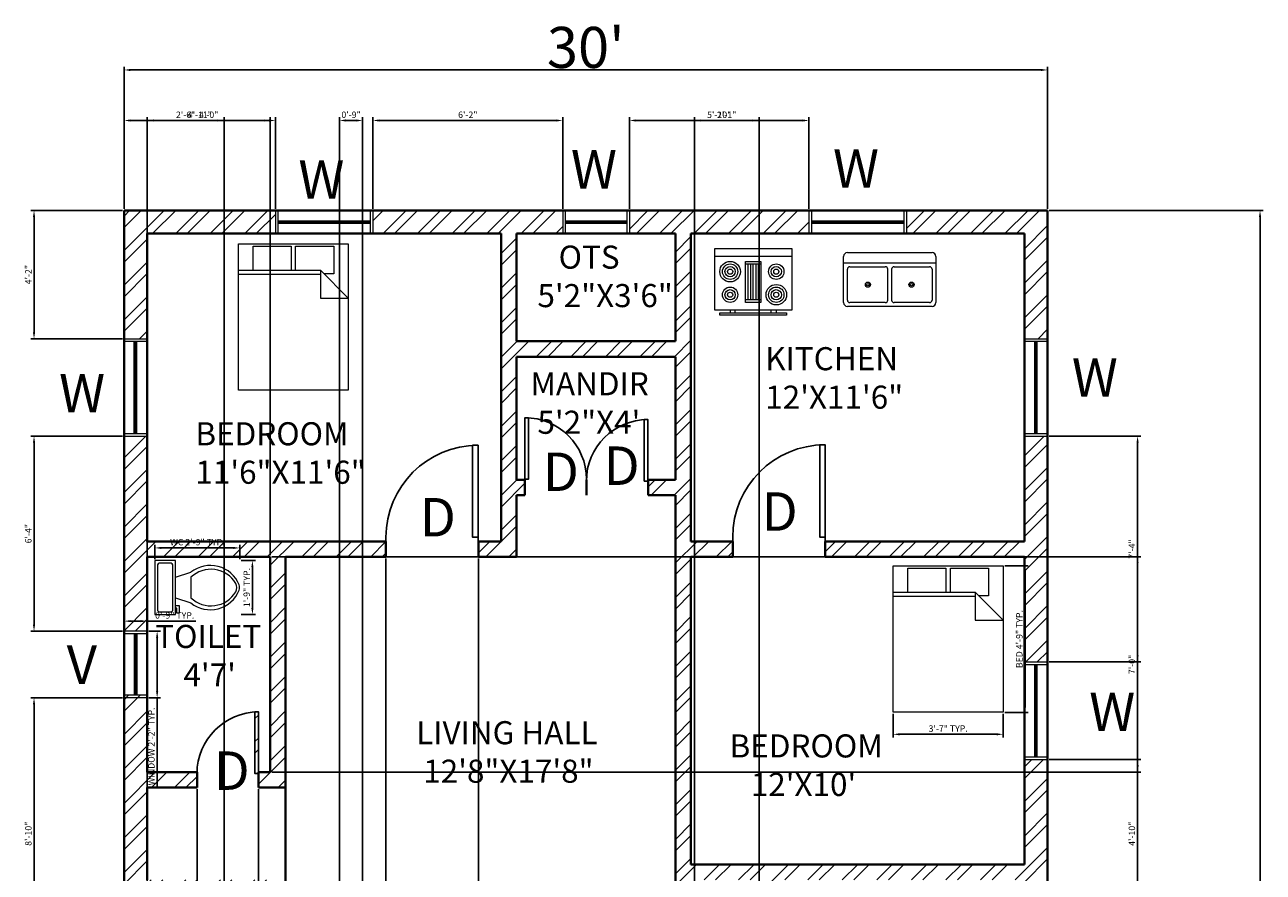
# Model space of a CAD drawing. Units: inches. Extents: x 1143 to 1626, y 7431 to 8140.
# Tile 4 of 4: x 1143 to 1626, y 7809 to 8140. Entities that reach past the tile are written whole.
import ezdxf

# ---------------------------------------------------------------- set-up
doc = ezdxf.new("R2010")
doc.units = ezdxf.units.IN
for name, color, linetype, lineweight in [('A-ANNO-DIMS', 4, 'Continuous', 18), ('A-DOOR', 3, 'Continuous', 25), ('A-GLAZ', 4, 'Continuous', 18), ('A-WALL', 2, 'Continuous', 40), ('A-WALL-PATT', 7, 'Continuous', 13)]:
    doc.layers.add(name, color=color, linetype=linetype, lineweight=lineweight)
for name, color, linetype, lineweight, true_color in [('A-ANNO-TEXT', 40, 'Continuous', 18, 0xf8d731), ('A-AREA-IDEN', 40, 'Continuous', 25, 0xf8d731), ('A-EQPM', 40, 'Continuous', 18, 0xf8d731), ('A-FLOR-FIXT', 40, 'Continuous', 18, 0xf8d731), ('A-FURN', 40, 'Continuous', 18, 0xf8d731)]:
    doc.layers.add(name, color=color, linetype=linetype, lineweight=lineweight, true_color=true_color)
doc.styles.get("Standard").update_dxf_attribs({"font": 'arial.ttf'})
doc.dimstyles.new('ISO-25', dxfattribs={"dimtxt": 2.5, "dimasz": 2.5, "dimexe": 1.25, "dimexo": 0.625, "dimtad": 1, "dimdec": 0, "dimlunit": 3, "dimtxsty": 'Standard', "dimcen": 2.5, "dimadec": 0, "dimazin": 0, "dimtfac": 1, "dimtdec": 0, "dimtmove": 0, "dimatfit": 3, "dimfxl": 1, "dimarcsym": 0})

# ---------------------------------------------------------------- blocks, each defined once
blk = doc.blocks.new('*U8')
for p, q in [((0, 0), (0, -100)), ((750, 0), (750, -100))]:
    blk.add_line(p, q)
blk.add_lwpolyline([(0, 0), (0, 750), (43.75, 750), (43.75, 0)], close=True)
blk.add_arc((0, 0), 750, 0, 90)
blk = doc.blocks.new('Bed - Queen')
for p, q in [((0, -80.00003), (0, 0)), ((0, 0), (59.99999, 0)), ((59.99999, 0), (59.99999, -80.00003)), ((7.99999, -1.2), (28.79998, -1.2)), ((7.99999, -14.4), (7.99999, -1.2)), ((28.79998, -1.2), (28.79998, -14.4)), ((31.19999, -1.2), (51.99999, -1.2)), ((31.19999, -14.4), (31.19999, -1.2)), ((51.99999, -1.2), (51.99999, -16.4)), ((0, -14.4), (44.8, -14.4)), ((44.8, -16.8), (0, -16.8)), ((59.99999, -29.6), (44.8, -14.4)), ((44.8, -14.4), (44.8, -29.6)), ((51.99999, -16.4), (46.79936, -16.4)), ((44.8, -29.6), (59.99999, -29.6)), ((59.99999, -80.00003), (0, -80.00003))]:
    blk.add_line(p, q)
blk = doc.blocks.new('Toilet - top')
for p, q in [((9.5, -6), (9.5, -2)), ((-10, -8.5), (-8, -8.5)), ((-10, -9.5), (-10, -8.5)), ((-7, -9.5), (-10, -9.5)), ((-8, -8.5), (-8, -8)), ((-7, -8), (-7, -9.5)), ((-4, -8), (-6, -14)), ((4, -8), (6, -14)), ((4, -14), (-4, -14))]:
    blk.add_line(p, q)
blk.add_lwpolyline([(10.5, -8), (10.5, 0), (-10.5, 0), (-10.5, -8)], close=True)
for points in [[(-9.5, -2), (-9.5, -6)], [(8.5, -1), (-8.5, -1)], [(-8.5, -7), (8.5, -7)]]:
    blk.add_lwpolyline(points)
for centre, radius, start, end in [((-8.62, -1.88), 0.884, 81.8699, 188.1301), ((8.62, -1.88), 0.884, 351.8699, 98.1301), ((-8.62, -6.12), 0.884, 171.8699, 278.1301), ((8.62, -6.12), 0.884, 261.8699, 8.1301), ((3.52, -21.58), 12.17, 141.4691, 247.9714), ((4.2, -21.82), 11.33, 136.3677, 238.9468), ((-3.52, -21.58), 12.17, 292.0284, 38.5307), ((-4.2, -21.82), 11.33, 301.053, 43.6321), ((0, -27.88), 4, 245.7318, 294.2682), ((0, -29), 4, 254.8605, 285.1395)]:
    blk.add_arc(centre, radius, start, end)
blk = doc.blocks.new('Range-Oven - 30 in top')
for p, q in [((0, -3), (30, -3)), ((12, -6), (18, -6)), ((13, -20), (13, -6)), ((14, -6), (14, -20)), ((15, -20), (15, -6)), ((16, -6), (16, -20)), ((17, -20), (17, -6)), ((6, -24), (6, -25)), ((8, -25), (8, -24)), ((18, -20), (12, -20)), ((22, -25), (22, -24)), ((24, -24), (24, -25))]:
    blk.add_line(p, q)
for points in [[(0, -24), (0, 0), (30, 0), (30, -24)], [(12, -21), (12, -5), (18, -5), (18, -21)], [(2, -26), (2, -25), (28, -25), (28, -26)]]:
    blk.add_lwpolyline(points, close=True)
for centre, radius in [((6, -9), 4), ((6, -9), 3), ((6, -9), 2), ((6, -9), 1), ((24, -9), 3), ((24, -9), 2), ((24, -9), 1), ((24, -18), 4), ((6, -18), 3), ((6, -18), 2), ((6, -18), 1), ((24, -18), 3), ((24, -18), 2), ((24, -18), 1)]:
    blk.add_circle(centre, radius)
blk = doc.blocks.new('Sink-double - 36 in top')
for p, q in [((-18, -4), (18, -4)), ((-0.75, -18.5), (-0.75, -6.5)), ((0.75, -6.5), (0.75, -18.5))]:
    blk.add_line(p, q)
for points in [[(-16.5, 0), (16.5, 0)], [(-18, -19.5), (-18, -1.5)], [(18, -1.5), (18, -19.5)], [(-16.5, -18.5), (-16.5, -6.5)], [(-15.5, -5.5), (-1.75, -5.5)], [(1.75, -5.5), (15.5, -5.5)], [(16.5, -6.5), (16.5, -18.5)], [(16.5, -21), (-16.5, -21)], [(-1.75, -19.5), (-15.5, -19.5)], [(15.5, -19.5), (1.75, -19.5)]]:
    blk.add_lwpolyline(points)
for centre, radius in [((-8.5, -12.5), 1), ((-8.5, -12.5), 0.5), ((8.5, -12.5), 1), ((8.5, -12.5), 0.5)]:
    blk.add_circle(centre, radius)
for centre, radius, start, end in [((-16.5, -1.5), 1.5, 90, 180), ((16.5, -1.5), 1.5, 0, 90), ((-15.5, -6.5), 1, 90, 180), ((-1.75, -6.5), 1, 0, 90), ((1.75, -6.5), 1, 90, 180), ((15.5, -6.5), 1, 0, 90), ((-15.5, -18.5), 1, 180, 270), ((-1.75, -18.5), 1, 270, 0), ((1.75, -18.5), 1, 180, 270), ((15.5, -18.5), 1, 270, 0), ((-16.5, -19.5), 1.5, 180, 270), ((16.5, -19.5), 1.5, 270, 0)]:
    blk.add_arc(centre, radius, start, end)
blk = doc.blocks.new('*D58')
at = {"layer": 'A-ANNO-DIMS', "color": 0, "lineweight": -2, "transparency": 16777216}
for p, q in [((1181.85, 8068.02), (1181.85, 8123.44)), ((1184.35, 8122.19), (1539.35, 8122.19)), ((1541.85, 8068.02), (1541.85, 8123.44))]:
    blk.add_line(p, q, dxfattribs=at)
at = {"layer": 'A-ANNO-DIMS', "color": 0, "transparency": 16777216}
for points in [[(1184.35, 8122.61), (1184.35, 8121.77), (1181.85, 8122.19)], [(1539.35, 8122.61), (1539.35, 8121.77), (1541.85, 8122.19)]]:
    blk.add_solid(points, dxfattribs=at)
at = {"layer": 'Defpoints', "color": 0, "transparency": 16777216}
for p in [(1541.85, 8122.19), (1181.85, 8067.4), (1541.85, 8067.4)]:
    blk.add_point(p, dxfattribs=at)
at = {"layer": 'A-ANNO-DIMS', "color": 0, "transparency": 16777216, "insert": (1361.85, 8130.99), "char_height": 2.5, "attachment_point": 5}
blk.add_mtext("{\\H6.4x;30'}", dxfattribs=at)
blk = doc.blocks.new('*D59')
at = {"layer": 'A-ANNO-DIMS', "color": 0, "lineweight": -2, "transparency": 16777216}
for p, q in [((1542.48, 8067.4), (1625.93, 8067.4)), ((1624.68, 8064.9), (1624.68, 7469.9)), ((1542.48, 7467.4), (1625.93, 7467.4))]:
    blk.add_line(p, q, dxfattribs=at)
at = {"layer": 'A-ANNO-DIMS', "color": 0, "transparency": 16777216}
for points in [[(1624.27, 8064.9), (1625.1, 8064.9), (1624.68, 8067.4)], [(1624.27, 7469.9), (1625.1, 7469.9), (1624.68, 7467.4)]]:
    blk.add_solid(points, dxfattribs=at)
at = {"layer": 'Defpoints', "color": 0, "transparency": 16777216}
for p in [(1541.85, 8067.4), (1541.85, 7467.4), (1624.68, 7467.4)]:
    blk.add_point(p, dxfattribs=at)
at = {"layer": 'A-ANNO-DIMS', "color": 0, "transparency": 16777216, "insert": (1615.89, 7767.4), "char_height": 2.5, "attachment_point": 5, "rotation": 90}
blk.add_mtext("{\\H6.4x;50'}", dxfattribs=at)
blk = doc.blocks.new('WIN-36IN')
for p, q in [((0, 9), (0, 0)), ((1, 9), (1, 0)), ((1, 5), (37, 5)), ((37, 9), (37, 0)), ((38, 9), (38, 0)), ((1, 4.5), (37, 4.5)), ((1, 4), (37, 4))]:
    blk.add_line(p, q)
blk = doc.blocks.new('WIN-24IN')
for p, q in [((0, 9), (0, 0)), ((1, 9), (1, 0)), ((1, 5), (25, 5)), ((25, 9), (25, 0)), ((26, 9), (26, 0)), ((1, 4.5), (25, 4.5)), ((1, 4), (25, 4))]:
    blk.add_line(p, q)
blk = doc.blocks.new('*D64')
at = {"layer": 'A-ANNO-DIMS', "color": 0, "lineweight": -2, "transparency": 16777216}
for p, q in [((1191.48, 7903.4), (1196, 7903.4)), ((1194.75, 7900.9), (1194.75, 7879.9)), ((1191.48, 7877.4), (1196, 7877.4)), ((1194.75, 7877.4), (1194.75, 7842.01))]:
    blk.add_line(p, q, dxfattribs=at)
at = {"layer": 'A-ANNO-DIMS', "color": 0, "transparency": 16777216}
for points in [[(1194.33, 7900.9), (1195.17, 7900.9), (1194.75, 7903.4)], [(1194.33, 7879.9), (1195.17, 7879.9), (1194.75, 7877.4)]]:
    blk.add_solid(points, dxfattribs=at)
at = {"layer": 'Defpoints', "color": 0, "transparency": 16777216}
for p in [(1190.85, 7903.4), (1190.85, 7877.4), (1194.75, 7877.4)]:
    blk.add_point(p, dxfattribs=at)
at = {"layer": 'A-ANNO-DIMS', "color": 0, "transparency": 16777216, "insert": (1192.83, 7858.45), "char_height": 2.5, "attachment_point": 5, "rotation": 90}
blk.add_mtext('WINDOW 2\'-2" TYP.', dxfattribs=at)
blk = doc.blocks.new('*D65')
at = {"layer": 'A-ANNO-DIMS', "color": 0, "lineweight": -2, "transparency": 16777216}
for p, q in [((1181.85, 7904.02), (1181.85, 7908.55)), ((1190.85, 7904.02), (1190.85, 7908.55)), ((1184.35, 7907.3), (1188.35, 7907.3)), ((1190.85, 7907.3), (1209.84, 7907.3))]:
    blk.add_line(p, q, dxfattribs=at)
at = {"layer": 'A-ANNO-DIMS', "color": 0, "transparency": 16777216}
for points in [[(1184.35, 7907.71), (1184.35, 7906.88), (1181.85, 7907.3)], [(1188.35, 7907.71), (1188.35, 7906.88), (1190.85, 7907.3)]]:
    blk.add_solid(points, dxfattribs=at)
at = {"layer": 'Defpoints', "color": 0, "transparency": 16777216}
for p in [(1181.85, 7903.4), (1190.85, 7907.3), (1190.85, 7903.4)]:
    blk.add_point(p, dxfattribs=at)
at = {"layer": 'A-ANNO-DIMS', "color": 0, "transparency": 16777216, "insert": (1201.59, 7909.2), "char_height": 2.5, "attachment_point": 5}
blk.add_mtext('0\'-9" TYP.', dxfattribs=at)
blk = doc.blocks.new('*D66')
at = {"layer": 'A-ANNO-DIMS', "color": 0, "lineweight": -2, "transparency": 16777216}
for p, q in [((1193.88, 7931.51), (1193.88, 7937.09)), ((1226.93, 7931.51), (1226.93, 7937.09)), ((1224.43, 7935.84), (1196.38, 7935.84))]:
    blk.add_line(p, q, dxfattribs=at)
at = {"layer": 'A-ANNO-DIMS', "color": 0, "transparency": 16777216}
for points in [[(1196.38, 7936.26), (1196.38, 7935.42), (1193.88, 7935.84)], [(1224.43, 7936.26), (1224.43, 7935.42), (1226.93, 7935.84)]]:
    blk.add_solid(points, dxfattribs=at)
at = {"layer": 'Defpoints', "color": 0, "transparency": 16777216}
for p in [(1193.88, 7935.84), (1193.88, 7930.88), (1226.93, 7930.88)]:
    blk.add_point(p, dxfattribs=at)
at = {"layer": 'A-ANNO-DIMS', "color": 0, "transparency": 16777216, "insert": (1210.41, 7937.76), "char_height": 2.5, "attachment_point": 5}
blk.add_mtext('WC 2\'-9" TYP.', dxfattribs=at)
blk = doc.blocks.new('*D67')
at = {"layer": 'A-ANNO-DIMS', "color": 0, "lineweight": -2, "transparency": 16777216}
for p, q in [((1227.56, 7930.88), (1233.14, 7930.88)), ((1231.89, 7912.38), (1231.89, 7928.38)), ((1227.56, 7909.88), (1233.14, 7909.88))]:
    blk.add_line(p, q, dxfattribs=at)
at = {"layer": 'A-ANNO-DIMS', "color": 0, "transparency": 16777216}
for points in [[(1231.47, 7928.38), (1232.3, 7928.38), (1231.89, 7930.88)], [(1231.47, 7912.38), (1232.3, 7912.38), (1231.89, 7909.88)]]:
    blk.add_solid(points, dxfattribs=at)
at = {"layer": 'Defpoints', "color": 0, "transparency": 16777216}
for p in [(1226.93, 7930.88), (1231.89, 7930.88), (1226.93, 7909.88)]:
    blk.add_point(p, dxfattribs=at)
at = {"layer": 'A-ANNO-DIMS', "color": 0, "transparency": 16777216, "insert": (1229.99, 7920.38), "char_height": 2.5, "attachment_point": 5, "rotation": 90}
blk.add_mtext('1\'-9" TYP.', dxfattribs=at)
blk = doc.blocks.new('*D68')
at = {"layer": 'A-ANNO-DIMS', "color": 0, "lineweight": -2, "transparency": 16777216}
for p, q in [((1525.14, 7928.84), (1534.33, 7928.84)), ((1533.08, 7874.24), (1533.08, 7926.34)), ((1525.14, 7871.74), (1534.33, 7871.74))]:
    blk.add_line(p, q, dxfattribs=at)
at = {"layer": 'A-ANNO-DIMS', "color": 0, "transparency": 16777216}
for points in [[(1532.67, 7926.34), (1533.5, 7926.34), (1533.08, 7928.84)], [(1532.67, 7874.24), (1533.5, 7874.24), (1533.08, 7871.74)]]:
    blk.add_solid(points, dxfattribs=at)
at = {"layer": 'Defpoints', "color": 0, "transparency": 16777216}
for p in [(1524.52, 7928.84), (1533.08, 7928.84), (1524.52, 7871.74)]:
    blk.add_point(p, dxfattribs=at)
at = {"layer": 'A-ANNO-DIMS', "color": 0, "transparency": 16777216, "insert": (1531.18, 7900.29), "char_height": 2.5, "attachment_point": 5, "rotation": 90}
blk.add_mtext('BED 4\'-9" TYP.', dxfattribs=at)
blk = doc.blocks.new('*D69')
at = {"layer": 'A-ANNO-DIMS', "color": 0, "lineweight": -2, "transparency": 16777216}
for p, q in [((1481.7, 7871.12), (1481.7, 7861.93)), ((1524.52, 7871.12), (1524.52, 7861.93)), ((1484.2, 7863.18), (1522.02, 7863.18))]:
    blk.add_line(p, q, dxfattribs=at)
at = {"layer": 'A-ANNO-DIMS', "color": 0, "transparency": 16777216}
for points in [[(1484.2, 7863.6), (1484.2, 7862.76), (1481.7, 7863.18)], [(1522.02, 7863.6), (1522.02, 7862.76), (1524.52, 7863.18)]]:
    blk.add_solid(points, dxfattribs=at)
at = {"layer": 'Defpoints', "color": 0, "transparency": 16777216}
for p in [(1481.7, 7871.74), (1524.52, 7871.74), (1524.52, 7863.18)]:
    blk.add_point(p, dxfattribs=at)
at = {"layer": 'A-ANNO-DIMS', "color": 0, "transparency": 16777216, "insert": (1503.11, 7865.08), "char_height": 2.5, "attachment_point": 5}
blk.add_mtext('3\'-7" TYP.', dxfattribs=at)
blk = doc.blocks.new('*D85')
at = {"layer": 'A-ANNO-DIMS', "color": 0, "lineweight": -2, "transparency": 16777216}
for p, q in [((1283.96, 7931.77), (1283.96, 7431.05)), ((1319.96, 7931.77), (1319.96, 7431.05)), ((1286.46, 7432.3), (1317.46, 7432.3))]:
    blk.add_line(p, q, dxfattribs=at)
at = {"layer": 'A-ANNO-DIMS', "color": 0, "transparency": 16777216}
for points in [[(1286.46, 7432.71), (1286.46, 7431.88), (1283.96, 7432.3)], [(1317.46, 7432.71), (1317.46, 7431.88), (1319.96, 7432.3)]]:
    blk.add_solid(points, dxfattribs=at)
at = {"layer": 'Defpoints', "color": 0, "transparency": 16777216}
for p in [(1283.96, 7932.4), (1319.96, 7932.4), (1319.96, 7432.3)]:
    blk.add_point(p, dxfattribs=at)
at = {"layer": 'A-ANNO-DIMS', "color": 0, "transparency": 16777216, "insert": (1301.96, 7434.2), "char_height": 2.5, "attachment_point": 5}
blk.add_mtext('3\'-0"', dxfattribs=at)
blk = doc.blocks.new('*D86')
at = {"layer": 'A-ANNO-DIMS', "color": 0, "lineweight": -2, "transparency": 16777216}
for p, q in [((1210.31, 7841.77), (1210.31, 7431.05)), ((1234.31, 7841.77), (1234.31, 7431.05)), ((1212.81, 7432.3), (1231.81, 7432.3))]:
    blk.add_line(p, q, dxfattribs=at)
at = {"layer": 'A-ANNO-DIMS', "color": 0, "transparency": 16777216}
for points in [[(1212.81, 7432.71), (1212.81, 7431.88), (1210.31, 7432.3)], [(1231.81, 7432.71), (1231.81, 7431.88), (1234.31, 7432.3)]]:
    blk.add_solid(points, dxfattribs=at)
at = {"layer": 'Defpoints', "color": 0, "transparency": 16777216}
for p in [(1210.31, 7842.4), (1234.31, 7842.4), (1234.31, 7432.3)]:
    blk.add_point(p, dxfattribs=at)
at = {"layer": 'A-ANNO-DIMS', "color": 0, "transparency": 16777216, "insert": (1222.31, 7434.2), "char_height": 2.5, "attachment_point": 5}
blk.add_mtext('2\'-0"', dxfattribs=at)
blk = doc.blocks.new('*D87')
at = {"layer": 'A-ANNO-DIMS', "color": 0, "lineweight": -2, "transparency": 16777216}
for p, q in [((1181.85, 8068.02), (1181.85, 8103.75)), ((1184.35, 8102.5), (1238.35, 8102.5)), ((1240.85, 8068.02), (1240.85, 8103.75))]:
    blk.add_line(p, q, dxfattribs=at)
at = {"layer": 'A-ANNO-DIMS', "color": 0, "transparency": 16777216}
for points in [[(1184.35, 8102.91), (1184.35, 8102.08), (1181.85, 8102.5)], [(1238.35, 8102.91), (1238.35, 8102.08), (1240.85, 8102.5)]]:
    blk.add_solid(points, dxfattribs=at)
at = {"layer": 'Defpoints', "color": 0, "transparency": 16777216}
for p in [(1240.85, 8102.5), (1181.85, 8067.4), (1240.85, 8067.4)]:
    blk.add_point(p, dxfattribs=at)
at = {"layer": 'A-ANNO-DIMS', "color": 0, "transparency": 16777216, "insert": (1211.35, 8104.38), "char_height": 2.5, "attachment_point": 5}
blk.add_mtext('4\'-11"', dxfattribs=at)
blk = doc.blocks.new('*D88')
at = {"layer": 'A-ANNO-DIMS', "color": 0, "lineweight": -2, "transparency": 16777216}
for p, q in [((1278.85, 8068.02), (1278.85, 8103.75)), ((1281.35, 8102.5), (1350.35, 8102.5)), ((1352.85, 8068.02), (1352.85, 8103.75))]:
    blk.add_line(p, q, dxfattribs=at)
at = {"layer": 'A-ANNO-DIMS', "color": 0, "transparency": 16777216}
for points in [[(1281.35, 8102.91), (1281.35, 8102.08), (1278.85, 8102.5)], [(1350.35, 8102.91), (1350.35, 8102.08), (1352.85, 8102.5)]]:
    blk.add_solid(points, dxfattribs=at)
at = {"layer": 'Defpoints', "color": 0, "transparency": 16777216}
for p in [(1352.85, 8102.5), (1278.85, 8067.4), (1352.85, 8067.4)]:
    blk.add_point(p, dxfattribs=at)
at = {"layer": 'A-ANNO-DIMS', "color": 0, "transparency": 16777216, "insert": (1315.85, 8104.4), "char_height": 2.5, "attachment_point": 5}
blk.add_mtext('6\'-2"', dxfattribs=at)
blk = doc.blocks.new('*D89')
at = {"layer": 'A-ANNO-DIMS', "color": 0, "lineweight": -2, "transparency": 16777216}
for p, q in [((1378.85, 8068.02), (1378.85, 8103.75)), ((1381.35, 8102.5), (1446.35, 8102.5)), ((1448.85, 8068.02), (1448.85, 8103.75))]:
    blk.add_line(p, q, dxfattribs=at)
at = {"layer": 'A-ANNO-DIMS', "color": 0, "transparency": 16777216}
for points in [[(1381.35, 8102.91), (1381.35, 8102.08), (1378.85, 8102.5)], [(1446.35, 8102.91), (1446.35, 8102.08), (1448.85, 8102.5)]]:
    blk.add_solid(points, dxfattribs=at)
at = {"layer": 'Defpoints', "color": 0, "transparency": 16777216}
for p in [(1448.85, 8102.5), (1378.85, 8067.4), (1448.85, 8067.4)]:
    blk.add_point(p, dxfattribs=at)
at = {"layer": 'A-ANNO-DIMS', "color": 0, "transparency": 16777216, "insert": (1413.85, 8104.4), "char_height": 2.5, "attachment_point": 5}
blk.add_mtext('5\'-10"', dxfattribs=at)
blk = doc.blocks.new('*D90')
at = {"layer": 'A-ANNO-DIMS', "color": 0, "lineweight": -2, "transparency": 16777216}
for p, q in [((1181.23, 8067.4), (1145.5, 8067.4)), ((1146.75, 8019.9), (1146.75, 8064.9)), ((1181.23, 8017.4), (1145.5, 8017.4))]:
    blk.add_line(p, q, dxfattribs=at)
at = {"layer": 'A-ANNO-DIMS', "color": 0, "transparency": 16777216}
for points in [[(1146.33, 8064.9), (1147.17, 8064.9), (1146.75, 8067.4)], [(1146.33, 8019.9), (1147.17, 8019.9), (1146.75, 8017.4)]]:
    blk.add_solid(points, dxfattribs=at)
at = {"layer": 'Defpoints', "color": 0, "transparency": 16777216}
for p in [(1146.75, 8067.4), (1181.85, 8067.4), (1181.85, 8017.4)]:
    blk.add_point(p, dxfattribs=at)
at = {"layer": 'A-ANNO-DIMS', "color": 0, "transparency": 16777216, "insert": (1144.87, 8042.4), "char_height": 2.5, "attachment_point": 5, "rotation": 90}
blk.add_mtext('4\'-2"', dxfattribs=at)
blk = doc.blocks.new('*D92')
at = {"layer": 'A-ANNO-DIMS', "color": 0, "lineweight": -2, "transparency": 16777216}
for p, q in [((1181.23, 7877.4), (1145.5, 7877.4)), ((1146.75, 7773.9), (1146.75, 7874.9)), ((1181.23, 7771.4), (1145.5, 7771.4))]:
    blk.add_line(p, q, dxfattribs=at)
at = {"layer": 'A-ANNO-DIMS', "color": 0, "transparency": 16777216}
for points in [[(1146.33, 7874.9), (1147.17, 7874.9), (1146.75, 7877.4)], [(1146.33, 7773.9), (1147.17, 7773.9), (1146.75, 7771.4)]]:
    blk.add_solid(points, dxfattribs=at)
at = {"layer": 'Defpoints', "color": 0, "transparency": 16777216}
for p in [(1146.75, 7877.4), (1181.85, 7877.4), (1181.85, 7771.4)]:
    blk.add_point(p, dxfattribs=at)
at = {"layer": 'A-ANNO-DIMS', "color": 0, "transparency": 16777216, "insert": (1144.85, 7824.4), "char_height": 2.5, "attachment_point": 5, "rotation": 90}
blk.add_mtext('8\'-10"', dxfattribs=at)
blk = doc.blocks.new('*D93')
at = {"layer": 'A-ANNO-DIMS', "color": 0, "lineweight": -2, "transparency": 16777216}
for p, q in [((1181.23, 7979.4), (1145.5, 7979.4)), ((1146.75, 7905.9), (1146.75, 7976.9)), ((1181.23, 7903.4), (1145.5, 7903.4))]:
    blk.add_line(p, q, dxfattribs=at)
at = {"layer": 'A-ANNO-DIMS', "color": 0, "transparency": 16777216}
for points in [[(1146.33, 7976.9), (1147.17, 7976.9), (1146.75, 7979.4)], [(1146.33, 7905.9), (1147.17, 7905.9), (1146.75, 7903.4)]]:
    blk.add_solid(points, dxfattribs=at)
at = {"layer": 'Defpoints', "color": 0, "transparency": 16777216}
for p in [(1146.75, 7979.4), (1181.85, 7979.4), (1181.85, 7903.4)]:
    blk.add_point(p, dxfattribs=at)
at = {"layer": 'A-ANNO-DIMS', "color": 0, "transparency": 16777216, "insert": (1144.85, 7941.4), "char_height": 2.5, "attachment_point": 5, "rotation": 90}
blk.add_mtext('6\'-4"', dxfattribs=at)
blk = doc.blocks.new('*D96')
at = {"layer": 'A-ANNO-DIMS', "color": 0, "lineweight": -2, "transparency": 16777216}
for p, q in [((1542.48, 7853.4), (1578.2, 7853.4)), ((1576.95, 7797.9), (1576.95, 7850.9)), ((1542.48, 7795.4), (1578.2, 7795.4))]:
    blk.add_line(p, q, dxfattribs=at)
at = {"layer": 'A-ANNO-DIMS', "color": 0, "transparency": 16777216}
for points in [[(1576.53, 7850.9), (1577.37, 7850.9), (1576.95, 7853.4)], [(1576.53, 7797.9), (1577.37, 7797.9), (1576.95, 7795.4)]]:
    blk.add_solid(points, dxfattribs=at)
at = {"layer": 'Defpoints', "color": 0, "transparency": 16777216}
for p in [(1541.85, 7853.4), (1576.95, 7853.4), (1541.85, 7795.4)]:
    blk.add_point(p, dxfattribs=at)
at = {"layer": 'A-ANNO-DIMS', "color": 0, "transparency": 16777216, "insert": (1575.05, 7824.4), "char_height": 2.5, "attachment_point": 5, "rotation": 90}
blk.add_mtext('4\'-10"', dxfattribs=at)
blk = doc.blocks.new('*D97')
at = {"layer": 'A-ANNO-DIMS', "color": 0, "lineweight": -2, "transparency": 16777216}
for p, q in [((1542.48, 7979.4), (1578.2, 7979.4)), ((1576.95, 7893.9), (1576.95, 7976.9)), ((1542.48, 7891.4), (1578.2, 7891.4))]:
    blk.add_line(p, q, dxfattribs=at)
at = {"layer": 'A-ANNO-DIMS', "color": 0, "transparency": 16777216}
for points in [[(1576.53, 7976.9), (1577.37, 7976.9), (1576.95, 7979.4)], [(1576.53, 7893.9), (1577.37, 7893.9), (1576.95, 7891.4)]]:
    blk.add_solid(points, dxfattribs=at)
at = {"layer": 'Defpoints', "color": 0, "transparency": 16777216}
for p in [(1541.85, 7979.4), (1576.95, 7979.4), (1541.85, 7891.4)]:
    blk.add_point(p, dxfattribs=at)
at = {"layer": 'A-ANNO-DIMS', "color": 0, "transparency": 16777216, "insert": (1575.08, 7935.4), "char_height": 2.5, "attachment_point": 5, "rotation": 90}
blk.add_mtext('7\'-4"', dxfattribs=at)
blk = doc.blocks.new('*D98')
at = {"layer": 'A-ANNO-DIMS', "color": 0, "lineweight": -2, "transparency": 16777216}
for p, q in [((1190.85, 7477.02), (1190.85, 8103.75)), ((1193.35, 8102.5), (1218.35, 8102.5)), ((1220.85, 7477.02), (1220.85, 8103.75))]:
    blk.add_line(p, q, dxfattribs=at)
at = {"layer": 'A-ANNO-DIMS', "color": 0, "transparency": 16777216}
for points in [[(1193.35, 8102.91), (1193.35, 8102.08), (1190.85, 8102.5)], [(1218.35, 8102.91), (1218.35, 8102.08), (1220.85, 8102.5)]]:
    blk.add_solid(points, dxfattribs=at)
at = {"layer": 'Defpoints', "color": 0, "transparency": 16777216}
for p in [(1220.85, 8102.5), (1190.85, 7476.4), (1220.85, 7476.4)]:
    blk.add_point(p, dxfattribs=at)
at = {"layer": 'A-ANNO-DIMS', "color": 0, "transparency": 16777216, "insert": (1205.85, 8104.4), "char_height": 2.5, "attachment_point": 5}
blk.add_mtext('2\'-6"', dxfattribs=at)
blk = doc.blocks.new('*D99')
at = {"layer": 'A-ANNO-DIMS', "color": 0, "lineweight": -2, "transparency": 16777216}
for p, q in [((1265.85, 7477.02), (1265.85, 8103.75)), ((1268.35, 8102.5), (1272.35, 8102.5)), ((1274.85, 7477.02), (1274.85, 8103.75))]:
    blk.add_line(p, q, dxfattribs=at)
at = {"layer": 'A-ANNO-DIMS', "color": 0, "transparency": 16777216}
for points in [[(1268.35, 8102.91), (1268.35, 8102.08), (1265.85, 8102.5)], [(1272.35, 8102.91), (1272.35, 8102.08), (1274.85, 8102.5)]]:
    blk.add_solid(points, dxfattribs=at)
at = {"layer": 'Defpoints', "color": 0, "transparency": 16777216}
for p in [(1274.85, 8102.5), (1265.85, 7476.4), (1274.85, 7476.4)]:
    blk.add_point(p, dxfattribs=at)
at = {"layer": 'A-ANNO-DIMS', "color": 0, "transparency": 16777216, "insert": (1270.35, 8104.4), "char_height": 2.5, "attachment_point": 5}
blk.add_mtext('0\'-9"', dxfattribs=at)
blk = doc.blocks.new('*D100')
at = {"layer": 'A-ANNO-DIMS', "color": 0, "lineweight": -2, "transparency": 16777216}
for p, q in [((1190.85, 7933.02), (1190.85, 8103.75)), ((1193.35, 8102.5), (1236.35, 8102.5)), ((1238.85, 7933.02), (1238.85, 8103.75))]:
    blk.add_line(p, q, dxfattribs=at)
at = {"layer": 'A-ANNO-DIMS', "color": 0, "transparency": 16777216}
for points in [[(1193.35, 8102.91), (1193.35, 8102.08), (1190.85, 8102.5)], [(1236.35, 8102.91), (1236.35, 8102.08), (1238.85, 8102.5)]]:
    blk.add_solid(points, dxfattribs=at)
at = {"layer": 'Defpoints', "color": 0, "transparency": 16777216}
for p in [(1238.85, 8102.5), (1190.85, 7932.4), (1238.85, 7932.4)]:
    blk.add_point(p, dxfattribs=at)
at = {"layer": 'A-ANNO-DIMS', "color": 0, "transparency": 16777216, "insert": (1214.85, 8104.4), "char_height": 2.5, "attachment_point": 5}
blk.add_mtext('4\'-0"', dxfattribs=at)
blk = doc.blocks.new('*D101')
at = {"layer": 'A-ANNO-DIMS', "color": 0, "lineweight": -2, "transparency": 16777216}
for p, q in [((1239.48, 7932.4), (1578.2, 7932.4)), ((1576.95, 7850.9), (1576.95, 7929.9)), ((1239.48, 7848.4), (1578.2, 7848.4))]:
    blk.add_line(p, q, dxfattribs=at)
at = {"layer": 'A-ANNO-DIMS', "color": 0, "transparency": 16777216}
for points in [[(1576.53, 7929.9), (1577.37, 7929.9), (1576.95, 7932.4)], [(1576.53, 7850.9), (1577.37, 7850.9), (1576.95, 7848.4)]]:
    blk.add_solid(points, dxfattribs=at)
at = {"layer": 'Defpoints', "color": 0, "transparency": 16777216}
for p in [(1238.85, 7932.4), (1576.95, 7932.4), (1238.85, 7848.4)]:
    blk.add_point(p, dxfattribs=at)
at = {"layer": 'A-ANNO-DIMS', "color": 0, "transparency": 16777216, "insert": (1575.05, 7890.4), "char_height": 2.5, "attachment_point": 5, "rotation": 90}
blk.add_mtext('7\'-0"', dxfattribs=at)
blk = doc.blocks.new('*D102')
at = {"layer": 'A-ANNO-DIMS', "color": 0, "lineweight": -2, "transparency": 16777216}
for p, q in [((1404.17, 7663.02), (1404.17, 8103.75)), ((1406.67, 8102.5), (1426.88, 8102.5)), ((1429.38, 7663.02), (1429.38, 8103.75))]:
    blk.add_line(p, q, dxfattribs=at)
at = {"layer": 'A-ANNO-DIMS', "color": 0, "transparency": 16777216}
for points in [[(1406.67, 8102.91), (1406.67, 8102.08), (1404.17, 8102.5)], [(1426.88, 8102.91), (1426.88, 8102.08), (1429.38, 8102.5)]]:
    blk.add_solid(points, dxfattribs=at)
at = {"layer": 'Defpoints', "color": 0, "transparency": 16777216}
for p in [(1429.38, 8102.5), (1404.17, 7662.4), (1429.38, 7662.4)]:
    blk.add_point(p, dxfattribs=at)
at = {"layer": 'A-ANNO-DIMS', "color": 0, "transparency": 16777216, "insert": (1416.78, 8104.38), "char_height": 2.5, "attachment_point": 5}
blk.add_mtext('2\'-1"', dxfattribs=at)

msp = doc.modelspace()

# ---------------------------------------------------------------- hatches: boundary and pattern name
at = {"layer": 'A-WALL-PATT'}
h = msp.add_hatch(dxfattribs=at)
h.set_pattern_fill('ANSI32', color=256)
h.paths.add_polyline_path([(1240.85, 8067.4), (1181.85, 8067.4), (1181.85, 8017.4), (1190.85, 8017.4), (1190.85, 8058.4), (1240.85, 8058.4)])
h.paths.add_polyline_path([(1541.85, 8067.4), (1486.85, 8067.4), (1486.85, 8058.4), (1532.85, 8058.4), (1532.85, 8017.4), (1541.85, 8017.4)], flags=17)
h.paths.add_polyline_path([(1352.85, 8067.4), (1278.85, 8067.4), (1278.85, 8058.4), (1328.85, 8058.4), (1328.85, 7938.4), (1319.96, 7938.4), (1319.96, 7932.4), (1334.85, 7932.4), (1334.85, 7956.4), (1338.11, 7956.4), (1338.11, 7962.4), (1334.85, 7962.4), (1334.85, 8010.4), (1396.85, 8010.4), (1396.85, 7962.4), (1386.11, 7962.4), (1386.11, 7956.4), (1396.85, 7956.4), (1396.85, 7662.4), (1393.24, 7662.4), (1393.24, 7656.4), (1404.17, 7656.4), (1404.17, 7662.4), (1402.85, 7662.4), (1402.85, 7806.4), (1430.85, 7806.4), (1430.85, 7786.73), (1436.85, 7786.73), (1436.85, 7806.4), (1532.85, 7806.4), (1532.85, 7795.4), (1541.85, 7795.4), (1541.85, 7853.4), (1532.85, 7853.4), (1532.85, 7812.4), (1402.85, 7812.4), (1402.85, 7932.4), (1419.12, 7932.4), (1419.12, 7938.4), (1402.85, 7938.4), (1402.85, 8058.4), (1448.85, 8058.4), (1448.85, 8067.4), (1378.85, 8067.4), (1378.85, 8058.4), (1396.85, 8058.4), (1396.85, 8016.4), (1334.85, 8016.4), (1334.85, 8058.4), (1352.85, 8058.4)])
h.paths.add_polyline_path([(1283.96, 7938.4), (1190.85, 7938.4), (1190.85, 7979.4), (1181.85, 7979.4), (1181.85, 7903.4), (1190.85, 7903.4), (1190.85, 7932.4), (1238.85, 7932.4), (1238.85, 7848.4), (1234.31, 7848.4), (1234.31, 7842.4), (1244.85, 7842.4), (1244.85, 7932.4), (1283.96, 7932.4)])
h.paths.add_polyline_path([(1541.85, 7979.4), (1532.85, 7979.4), (1532.85, 7938.4), (1455.12, 7938.4), (1455.12, 7932.4), (1532.85, 7932.4), (1532.85, 7891.4), (1541.85, 7891.4)], flags=17)
h.paths.add_polyline_path([(1210.81, 7716.4), (1190.85, 7716.4), (1190.85, 7745.4), (1181.85, 7745.4), (1181.85, 7663.4), (1190.85, 7663.4), (1190.85, 7710.4), (1210.81, 7710.4)])
h.paths.add_polyline_path([(1232.89, 7871.85), (1232.89, 7871.89), (1234.29, 7871.89), (1234.29, 7847.89), (1232.89, 7847.89), (1232.89, 7871.85, 0.385662), (1210.31, 7848.85), (1210.31, 7842.4), (1190.85, 7842.4), (1190.85, 7806.4), (1244.85, 7806.4), (1244.85, 7716.4), (1325.66, 7716.4), (1334.85, 7716.4), (1334.85, 7706.63), (1328.13, 7706.63), (1328.13, 7704.53), (1292.13, 7704.53), (1292.13, 7706.63), (1328.85, 7706.63), (1328.85, 7710.4), (1325.66, 7710.4), (1234.81, 7710.4), (1234.81, 7716.6), (1233.41, 7716.6), (1233.41, 7740.6), (1234.81, 7740.6), (1234.81, 7716.4), (1238.85, 7716.4), (1238.85, 7800.4), (1190.85, 7800.4), (1190.85, 7770.4), (1186.85, 7770.4), (1186.85, 7746.4), (1185.85, 7746.4), (1185.85, 7770.4), (1181.85, 7770.4), (1181.85, 7878.4), (1190.85, 7878.4), (1190.85, 7848.4), (1210.3, 7848.4, -0.391105)])
h.paths.add_polyline_path([(1541.85, 7688.4), (1532.85, 7688.4), (1532.85, 7662.4), (1436.85, 7662.4), (1436.85, 7712.56), (1430.85, 7712.56), (1430.85, 7662.4), (1429.38, 7656.4), (1532.85, 7656.4), (1532.85, 7467.4), (1541.85, 7467.4)])
h.paths.add_polyline_path([(1334.85, 7656.4), (1357.24, 7656.4), (1357.24, 7662.4), (1334.85, 7662.4), (1334.85, 7670.63), (1328.85, 7670.63), (1328.85, 7618.14), (1334.85, 7618.14)])
h.paths.add_polyline_path([(1190.85, 7572.4), (1334.85, 7572.4), (1334.85, 7582.14), (1328.85, 7582.14), (1328.85, 7578.4), (1190.85, 7578.4), (1190.85, 7625.4), (1181.85, 7625.4), (1181.85, 7467.4), (1324.72, 7467.4), (1324.72, 7476.4), (1190.85, 7476.4)])

# ---------------------------------------------------------------- linework, layer by layer
at = {"layer": 'A-WALL'}
for p, q in [((1181.85, 8067.4), (1541.85, 8067.4)), ((1181.85, 7467.4), (1181.85, 8067.4)), ((1541.85, 8067.4), (1541.85, 7467.4)), ((1190.85, 8058.4), (1328.85, 8058.4)), ((1190.85, 7938.4), (1190.85, 8058.4)), ((1328.85, 7938.4), (1328.85, 8058.4)), ((1334.85, 8016.4), (1334.85, 8058.4)), ((1334.85, 8058.4), (1396.85, 8058.4)), ((1396.85, 8016.4), (1396.85, 8058.4)), ((1402.85, 7938.4), (1402.85, 8058.4)), ((1402.85, 8058.4), (1532.85, 8058.4)), ((1532.85, 8058.4), (1532.85, 7938.4)), ((1334.85, 8016.4), (1396.85, 8016.4)), ((1334.85, 8010.4), (1396.85, 8010.4)), ((1334.85, 7962.4), (1334.85, 8010.4)), ((1396.85, 7962.4), (1396.85, 8010.4)), ((1334.85, 7962.4), (1338.11, 7962.4)), ((1338.11, 7962.4), (1338.11, 7956.4)), ((1362.11, 7962.4), (1362.11, 7956.4)), ((1386.11, 7962.4), (1386.11, 7956.4)), ((1386.11, 7962.4), (1396.85, 7962.4)), ((1334.85, 7932.4), (1334.85, 7956.4)), ((1334.85, 7956.4), (1338.11, 7956.4)), ((1386.11, 7956.4), (1396.85, 7956.4)), ((1396.85, 7662.4), (1396.85, 7956.4)), ((1190.85, 7938.4), (1283.96, 7938.4)), ((1283.96, 7938.4), (1283.96, 7932.4)), ((1319.96, 7938.4), (1319.96, 7932.4)), ((1319.96, 7938.4), (1328.85, 7938.4)), ((1402.85, 7938.4), (1419.12, 7938.4)), ((1419.12, 7938.4), (1419.12, 7932.4)), ((1455.12, 7938.4), (1455.12, 7932.4)), ((1455.12, 7938.4), (1532.85, 7938.4)), ((1190.85, 7932.4), (1238.85, 7932.4)), ((1190.85, 7848.4), (1190.85, 7932.4)), ((1238.85, 7848.4), (1238.85, 7932.4)), ((1244.85, 7716.4), (1244.85, 7932.4)), ((1244.85, 7932.4), (1283.96, 7932.4)), ((1319.96, 7932.4), (1334.85, 7932.4)), ((1402.85, 7932.4), (1419.12, 7932.4)), ((1402.85, 7812.4), (1402.85, 7932.4)), ((1455.12, 7932.4), (1532.85, 7932.4)), ((1532.85, 7932.4), (1532.85, 7812.4)), ((1190.85, 7848.4), (1210.31, 7848.4)), ((1210.31, 7848.4), (1210.31, 7842.4)), ((1234.31, 7848.4), (1234.31, 7842.4)), ((1234.31, 7848.4), (1238.85, 7848.4)), ((1190.85, 7842.4), (1210.31, 7842.4)), ((1190.85, 7806.4), (1190.85, 7842.4)), ((1234.31, 7842.4), (1244.85, 7842.4)), ((1402.85, 7812.4), (1532.85, 7812.4))]:
    msp.add_line(p, q, dxfattribs=at)

# ---------------------------------------------------------------- block references
at = {"layer": 'A-DOOR'}
for p, xscale, yscale, zscale in [((1338.11, 7962.6), 0.0320000000000002, 0.0320000000000002, 0.0320000000000002), ((1386.05, 7961.92), -0.0319465227634566, 0.0319465227634566, 0.0319465227634566), ((1319.83, 7939.98), -0.0478243873005274, 0.0478243873005274, 0.0478243873005274), ((1455.12, 7940.05), -0.0479976400052493, 0.0479976400052493, 0.0479976400052493), ((1234.29, 7847.89), -0.0320000000000001, 0.0320000000000001, 0.0320000000000001)]:
    msp.add_blockref('*U8', p, dxfattribs=dict(at, xscale=xscale, yscale=yscale, zscale=zscale))
at = {"layer": 'A-EQPM'}
msp.add_blockref('Range-Oven - 30 in top', (1412.11, 8052.56), dxfattribs=at)
at = {"layer": 'A-FLOR-FIXT'}
msp.add_blockref('Sink-double - 36 in top', (1480.33, 8050.99), dxfattribs=at)
at = {"layer": 'A-FLOR-FIXT', "rotation": 89.99999999999999}
msp.add_blockref('Toilet - top', (1193.88, 7920.38), dxfattribs=at)
at = {"layer": 'A-FURN', "xscale": 0.7137426440278095, "yscale": 0.7137426440278095, "zscale": 0.7137426440278095}
for p in [(1226.45, 8054.41), (1481.7, 7928.84)]:
    msp.add_blockref('Bed - Queen', p, dxfattribs=at)
at = {"layer": 'A-GLAZ'}
for name, p in [('WIN-36IN', (1240.85, 8058.4)), ('WIN-24IN', (1352.85, 8058.4)), ('WIN-36IN', (1448.85, 8058.4))]:
    msp.add_blockref(name, p, dxfattribs=at)
for name, p, rotation in [('WIN-36IN', (1190.85, 7979.4), 89.99999999999883), ('WIN-36IN', (1541.85, 7979.4), 89.99999999999692), ('WIN-24IN', (1181.85, 7903.4), 270.000000000001), ('WIN-36IN', (1541.85, 7853.4), 89.99999999999628)]:
    msp.add_blockref(name, p, dxfattribs=dict(at, rotation=rotation))

# ---------------------------------------------------------------- texts
at = {"layer": 'A-ANNO-TEXT', "char_height": 15, "attachment_point": 1}
for s, insert in [('{W}', (1249.79, 8087.01)), ('{W}', (1356.04, 8090.96)), ('{W}', (1458.2, 8091.31)), ('{W}', (1551.31, 8009.82)), ('{W}', (1156.51, 8003.65)), ('{D}', (1345.08, 7973.03)), ('{D}', (1368.77, 7975.39)), ('{D}', (1430.39, 7957.53)), ('{D}', (1297.12, 7955.32)), ('{V}', (1159.51, 7897.81)), ('{W}', (1558.08, 7879.4)), ('{D}', (1216.74, 7856.51))]:
    msp.add_mtext_dynamic_manual_height_columns(s, width=1087.9578, gutter_width=12.5, heights=[0], dxfattribs=dict(at, insert=insert))
at = {"layer": 'A-AREA-IDEN', "char_height": 9, "attachment_point": 1}
for s, insert in [('{     OTS\\P  5\'2"X3\'6"}', (1337.5, 8053.72)), ('{KITCHEN\\P12\'X11\'6"}', (1431.8, 8014.12)), ('{ MANDIR\\P  5\'2"X4\'}', (1337.5, 8004.34)), ('{BEDROOM\\P11\'6"X11\'6"}', (1209.65, 7984.85)), ("{  TOILET\\P      4'7'}", (1188.5, 7905.83)), ('{LIVING HALL\\P 12\'8"X17\'8"}', (1295.73, 7868.29)), ("{BEDROOM\\P   12'X10'}", (1417.9, 7863.14))]:
    msp.add_mtext_dynamic_manual_height_columns(s, width=1087.9578, gutter_width=12.5, heights=[0], dxfattribs=dict(at, insert=insert))

# ---------------------------------------------------------------- dimensions: what is measured, and where the dimension line sits
at = {"layer": 'A-ANNO-DIMS'}
for base, p1, p2, text, override, picture, middle in [((1541.85, 8122.19), (1181.85, 8067.4), (1541.85, 8067.4), '{\\H6.4x;<>}', {"dimclrd": 0, "dimclre": 0, "dimclrt": 0}, '*D58', (1361.85, 8130.99)), ((1190.85, 7907.3), (1181.85, 7903.4), (1190.85, 7903.4), '<> TYP.', {"dimdec": 1, "dimlfac": 1, "dimrnd": 0, "dimzin": 1, "dimdsep": 46, "dimlunit": 4, "dimfrac": 2}, '*D65', (1201.59, 7909.2)), ((1524.52, 7863.18), (1481.7, 7871.74), (1524.52, 7871.74), '<> TYP.', {"dimdec": 1, "dimlfac": 1, "dimrnd": 0, "dimzin": 1, "dimdsep": 46, "dimlunit": 4, "dimfrac": 2}, '*D69', (1503.11, 7865.08))]:
    dim = msp.add_linear_dim(base=base, p1=p1, p2=p2, text=text, dimstyle='ISO-25', override=override, dxfattribs=at)
    dim.commit()
    dim.dimension.update_dxf_attribs({"geometry": picture, "text_midpoint": middle})
for base, p1, p2, picture, middle in [((1240.85, 8102.5), (1181.85, 8067.4), (1240.85, 8067.4), '*D87', (1211.35, 8104.38)), ((1220.85, 8102.5), (1190.85, 7476.4), (1220.85, 7476.4), '*D98', (1205.85, 8104.4)), ((1238.85, 8102.5), (1190.85, 7932.4), (1238.85, 7932.4), '*D100', (1214.85, 8104.4)), ((1274.85, 8102.5), (1265.85, 7476.4), (1274.85, 7476.4), '*D99', (1270.35, 8104.4)), ((1352.85, 8102.5), (1278.85, 8067.4), (1352.85, 8067.4), '*D88', (1315.85, 8104.4)), ((1448.85, 8102.5), (1378.85, 8067.4), (1448.85, 8067.4), '*D89', (1413.85, 8104.4)), ((1429.38, 8102.5), (1404.17, 7662.4), (1429.38, 7662.4), '*D102', (1416.78, 8104.38)), ((1319.96, 7432.3), (1283.96, 7932.4), (1319.96, 7932.4), '*D85', (1301.96, 7434.2)), ((1234.31, 7432.3), (1210.31, 7842.4), (1234.31, 7842.4), '*D86', (1222.31, 7434.2))]:
    dim = msp.add_linear_dim(base=base, p1=p1, p2=p2, dimstyle='ISO-25', override={"dimdec": 1, "dimlfac": 1, "dimrnd": 0, "dimzin": 1, "dimdsep": 46, "dimlunit": 4, "dimfrac": 2}, dxfattribs=at)
    dim.commit()
    dim.dimension.update_dxf_attribs({"geometry": picture, "text_midpoint": middle})
for base, p1, p2, picture, middle in [((1146.75, 8067.4), (1181.85, 8017.4), (1181.85, 8067.4), '*D90', (1144.87, 8042.4)), ((1146.75, 7979.4), (1181.85, 7903.4), (1181.85, 7979.4), '*D93', (1144.85, 7941.4)), ((1576.95, 7979.4), (1541.85, 7891.4), (1541.85, 7979.4), '*D97', (1575.08, 7935.4)), ((1576.95, 7932.4), (1238.85, 7848.4), (1238.85, 7932.4), '*D101', (1575.05, 7890.4)), ((1146.75, 7877.4), (1181.85, 7771.4), (1181.85, 7877.4), '*D92', (1144.85, 7824.4)), ((1576.95, 7853.4), (1541.85, 7795.4), (1541.85, 7853.4), '*D96', (1575.05, 7824.4))]:
    dim = msp.add_linear_dim(base=base, p1=p1, p2=p2, angle=90, dimstyle='ISO-25', override={"dimdec": 1, "dimlfac": 1, "dimrnd": 0, "dimzin": 1, "dimdsep": 46, "dimlunit": 4, "dimfrac": 2}, dxfattribs=at)
    dim.commit()
    dim.dimension.update_dxf_attribs({"geometry": picture, "text_midpoint": middle})
for base, p1, p2, angle, text, override, picture, middle in [((1624.68, 7467.4), (1541.85, 8067.4), (1541.85, 7467.4), 90, '{\\H6.4x;<>}', {"dimclrd": 0, "dimclre": 0, "dimclrt": 0}, '*D59', (1615.89, 7767.4)), ((1193.8849, 7935.8414), (1226.9311, 7930.8845), (1193.8849, 7930.8845), 180, 'WC <> TYP.', {"dimdec": 1, "dimlfac": 1, "dimrnd": 0, "dimzin": 1, "dimdsep": 46, "dimlunit": 4, "dimfrac": 2}, '*D66', (1210.408, 7937.7591)), ((1231.89, 7930.88), (1226.93, 7909.88), (1226.93, 7930.88), 90, '<> TYP.', {"dimdec": 1, "dimlfac": 1, "dimrnd": 0, "dimzin": 1, "dimdsep": 46, "dimlunit": 4, "dimfrac": 2}, '*D67', (1229.99, 7920.38)), ((1533.08, 7928.84), (1524.52, 7871.74), (1524.52, 7928.84), 90, 'BED <> TYP.', {"dimdec": 1, "dimlfac": 1, "dimrnd": 0, "dimzin": 1, "dimdsep": 46, "dimlunit": 4, "dimfrac": 2}, '*D68', (1531.18, 7900.29)), ((1194.75, 7877.4), (1190.85, 7903.4), (1190.85, 7877.4), 270, 'WINDOW <> TYP.', {"dimdec": 1, "dimlfac": 1, "dimrnd": 0, "dimzin": 1, "dimdsep": 46, "dimlunit": 4, "dimfrac": 2}, '*D64', (1192.83, 7858.45))]:
    dim = msp.add_linear_dim(base=base, p1=p1, p2=p2, angle=angle, text=text, dimstyle='ISO-25', override=override, dxfattribs=at)
    dim.commit()
    dim.dimension.update_dxf_attribs({"geometry": picture, "text_midpoint": middle})

doc.saveas('drawing.dxf')
